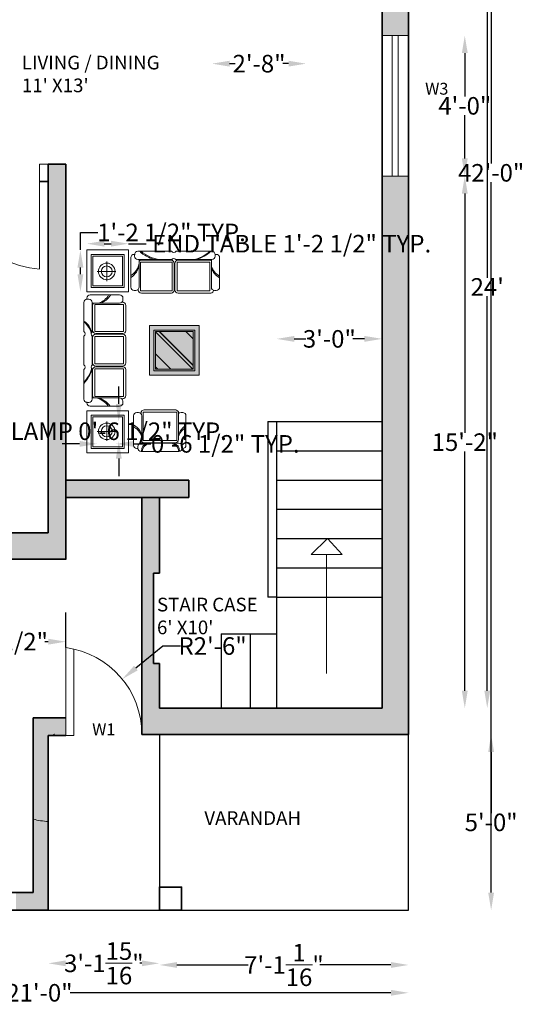
# Model space of a CAD drawing. Units: inches. Extents: x 2178 to 3409, y 1711 to 2279.
# Tile 2 of 8: x 2343 to 2516, y 1711 to 2047. Entities that reach past the tile are written whole.
import ezdxf

# ---------------------------------------------------------------- set-up
doc = ezdxf.new("R2010")
doc.units = ezdxf.units.IN
doc.linetypes.add('ACAD_ISO03W100', pattern=[30, 12, -18])
for name, color, linetype, lineweight in [('A-ANNO-DIMS', 2, 'Continuous', 18), ('A-ANNO-IDEN', 3, 'Continuous', 18), ('A-ANNO-SYMB', 7, 'Continuous', 18), ('A-AREA-IDEN', 7, 'Continuous', 18), ('A-COLS', 7, 'Continuous', 35), ('A-DOOR', 4, 'Continuous', 18), ('A-FLOR', 7, 'Continuous', 25), ('A-FLOR-STRS', 7, 'Continuous', 25), ('A-FURN', 8, 'Continuous', 18), ('A-FURN-PATT', 9, 'Continuous', 13), ('A-GLAZ', 4, 'Continuous', 18), ('A-WALL', 7, 'Continuous', 35), ('A-WALL-HIDN', 7, 'ACAD_ISO03W100', 25), ('A-WALL-PATT', 252, 'Continuous', 13)]:
    doc.layers.add(name, color=color, linetype=linetype, lineweight=lineweight)
doc.styles.get("Standard").update_dxf_attribs({"font": 'arial.ttf'})
doc.dimstyles.get("Standard").update_dxf_attribs({"dimtxt": 6, "dimasz": 6, "dimexe": 0.18, "dimexo": 0.0625, "dimgap": 0.09, "dimtad": 0, "dimtih": 1, "dimtoh": 1, "dimdec": 4, "dimzin": 0, "dimdsep": 46, "dimlunit": 4, "dimtxsty": 'Standard', "dimcen": 0.09, "dimse1": 1, "dimse2": 1, "dimadec": 0, "dimazin": 0, "dimtfac": 1, "dimtdec": 4, "dimtofl": 0, "dimtmove": 0, "dimatfit": 3, "dimfxl": 1, "dimtolj": 1, "dimtzin": 0, "dimarcsym": 0})

# ---------------------------------------------------------------- blocks, each defined once
blk = doc.blocks.new('*D17')
at = {"layer": 'A-ANNO-DIMS', "color": 0, "lineweight": -2, "transparency": 16777216}
for p, q in [((2359.06, 1724.86), (2359.75, 1724.86)), ((2385.03, 1724.86), (2384.35, 1724.86))]:
    blk.add_line(p, q, dxfattribs=at)
at = {"layer": 'A-ANNO-DIMS', "color": 0, "transparency": 16777216}
for points in [[(2359.06, 1725.86), (2359.06, 1723.86), (2353.06, 1724.86)], [(2385.03, 1725.86), (2385.03, 1723.86), (2391.03, 1724.86)]]:
    blk.add_solid(points, dxfattribs=at)
at = {"layer": 'Defpoints', "color": 0, "transparency": 16777216}
for p in [(2353.06, 1743.04), (2391.03, 1743.04), (2391.03, 1724.86)]:
    blk.add_point(p, dxfattribs=at)
at = {"layer": 'A-ANNO-DIMS', "color": 0, "transparency": 16777216, "insert": (2372.05, 1724.86), "char_height": 6, "attachment_point": 5}
blk.add_mtext('\\A1;3\'-1{\\H1x;\\S15/16;}"', dxfattribs=at)
blk = doc.blocks.new('*D18')
at = {"layer": 'A-ANNO-DIMS', "color": 0, "lineweight": -2, "transparency": 16777216}
for p, q in [((2397.03, 1724.3), (2421.29, 1724.3)), ((2470.06, 1724.3), (2445.8, 1724.3))]:
    blk.add_line(p, q, dxfattribs=at)
at = {"layer": 'A-ANNO-DIMS', "color": 0, "transparency": 16777216}
for points in [[(2397.03, 1725.3), (2397.03, 1723.3), (2391.03, 1724.3)], [(2470.06, 1725.3), (2470.06, 1723.3), (2476.06, 1724.3)]]:
    blk.add_solid(points, dxfattribs=at)
at = {"layer": 'Defpoints', "color": 0, "transparency": 16777216}
for p in [(2391.03, 1743.04), (2476.06, 1743.04), (2476.06, 1724.3)]:
    blk.add_point(p, dxfattribs=at)
at = {"layer": 'A-ANNO-DIMS', "color": 0, "transparency": 16777216, "insert": (2433.55, 1724.3), "char_height": 6, "attachment_point": 5}
blk.add_mtext('\\A1;7\'-1{\\H1x;\\S1/16;}"', dxfattribs=at)
blk = doc.blocks.new('*D22')
at = {"layer": 'A-ANNO-DIMS', "color": 0, "lineweight": -2, "transparency": 16777216}
for p, q in [((2502.98, 2094.04), (2502.98, 1959.14)), ((2502.98, 1818.04), (2502.98, 1952.94))]:
    blk.add_line(p, q, dxfattribs=at)
at = {"layer": 'A-ANNO-DIMS', "color": 0, "transparency": 16777216}
for points in [[(2501.98, 2094.04), (2503.98, 2094.04), (2502.98, 2100.04)], [(2501.98, 1818.04), (2503.98, 1818.04), (2502.98, 1812.04)]]:
    blk.add_solid(points, dxfattribs=at)
at = {"layer": 'Defpoints', "color": 0, "transparency": 16777216}
for p in [(2467.06, 2100.04), (2467.06, 1812.04), (2502.98, 1812.04)]:
    blk.add_point(p, dxfattribs=at)
at = {"layer": 'A-ANNO-DIMS', "color": 0, "transparency": 16777216, "insert": (2502.98, 1956.04), "char_height": 6, "attachment_point": 5}
blk.add_mtext("\\A1;24'", dxfattribs=at)
blk = doc.blocks.new('END-TABLE')
for p, q in [((14.32, 14.32), (0, 14.32)), ((0, 14.32), (0, 0)), ((14.32, 0), (14.32, 14.32)), ((12.81, 12.81), (1.51, 12.81)), ((1.51, 12.81), (1.51, 1.51)), ((12.25, 12.25), (2.07, 12.25)), ((2.07, 12.25), (2.07, 2.07)), ((12.25, 2.07), (12.25, 12.25)), ((12.81, 1.51), (12.81, 12.81)), ((0, 0), (14.32, 0)), ((1.51, 1.51), (12.81, 1.51)), ((2.07, 2.07), (12.25, 2.07))]:
    blk.add_line(p, q)
blk = doc.blocks.new('TABLE-LAMP')
for p, q in [((3.28, 0), (3.28, 6.65)), ((0, 3.28), (6.38, 3.28))]:
    blk.add_line(p, q)
for radius in [2.83, 1.88]:
    blk.add_circle((3.28, 3.28), radius)
blk = doc.blocks.new('DOOR-36')
for p, q in [((0, 0), (0, 36)), ((3, 0), (3, 35.87)), ((3, 0), (0, 0))]:
    blk.add_line(p, q)
blk.add_arc((0, 0), 36, 0, 85.2198)
blk = doc.blocks.new('*D43')
at = {"layer": 'A-ANNO-DIMS', "color": 0, "lineweight": -2, "transparency": 16777216}
for p, q in [((2372.2, 1970.82), (2374.52, 1970.82)), ((2380.52, 1970.82), (2386.52, 1970.82))]:
    blk.add_line(p, q, dxfattribs=at)
at = {"layer": 'A-ANNO-DIMS', "color": 0, "transparency": 16777216}
for points in [[(2372.2, 1971.82), (2372.2, 1969.82), (2366.2, 1970.82)], [(2374.52, 1971.82), (2374.52, 1969.82), (2380.52, 1970.82)]]:
    blk.add_solid(points, dxfattribs=at)
at = {"layer": 'Defpoints', "color": 0, "transparency": 16777216}
for p in [(2366.2, 1968.67), (2380.52, 1970.82), (2380.52, 1968.67)]:
    blk.add_point(p, dxfattribs=at)
at = {"layer": 'A-ANNO-DIMS', "color": 0, "transparency": 16777216, "insert": (2436.18, 1970.82), "char_height": 6, "attachment_point": 5}
blk.add_mtext('\\A1;END TABLE 1\'-2 1/2" TYP.', dxfattribs=at)
blk = doc.blocks.new('*D44')
at = {"layer": 'A-ANNO-DIMS', "color": 0, "lineweight": -2, "transparency": 16777216}
for p, q in [((2364.05, 1968.67), (2364.05, 1974.67)), ((2364.05, 1974.67), (2370.05, 1974.67)), ((2364.05, 1960.35), (2364.05, 1962.67))]:
    blk.add_line(p, q, dxfattribs=at)
at = {"layer": 'A-ANNO-DIMS', "color": 0, "transparency": 16777216}
for points in [[(2363.05, 1962.67), (2365.05, 1962.67), (2364.05, 1968.67)], [(2363.05, 1960.35), (2365.05, 1960.35), (2364.05, 1954.35)]]:
    blk.add_solid(points, dxfattribs=at)
at = {"layer": 'Defpoints', "color": 0, "transparency": 16777216}
for p in [(2364.05, 1968.67), (2366.2, 1968.67), (2366.2, 1954.35)]:
    blk.add_point(p, dxfattribs=at)
at = {"layer": 'A-ANNO-DIMS', "color": 0, "transparency": 16777216, "insert": (2395.14, 1974.67), "char_height": 6, "attachment_point": 5}
blk.add_mtext('\\A1;1\'-2 1/2" TYP.', dxfattribs=at)
blk = doc.blocks.new('*D45')
at = {"layer": 'A-ANNO-DIMS', "color": 0, "lineweight": -2, "transparency": 16777216}
for p, q in [((2377.15, 1916.05), (2377.15, 1922.05)), ((2377.15, 1897.4), (2377.15, 1891.4))]:
    blk.add_line(p, q, dxfattribs=at)
at = {"layer": 'A-ANNO-DIMS', "color": 0, "transparency": 16777216}
for points in [[(2376.15, 1916.05), (2378.15, 1916.05), (2377.15, 1910.05)], [(2376.15, 1897.4), (2378.15, 1897.4), (2377.15, 1903.4)]]:
    blk.add_solid(points, dxfattribs=at)
at = {"layer": 'Defpoints', "color": 0, "transparency": 16777216}
for p in [(2376.15, 1910.05), (2377.15, 1910.05), (2376.15, 1903.4)]:
    blk.add_point(p, dxfattribs=at)
at = {"layer": 'A-ANNO-DIMS', "color": 0, "transparency": 16777216, "insert": (2377.15, 1906.72), "char_height": 6, "attachment_point": 5}
blk.add_mtext('\\A1;LAMP 0\'-6 1/2" TYP.', dxfattribs=at)
blk = doc.blocks.new('*D46')
at = {"layer": 'A-ANNO-DIMS', "color": 0, "lineweight": -2, "transparency": 16777216}
for p, q in [((2363.77, 1902.4), (2357.77, 1902.4)), ((2382.15, 1902.4), (2388.15, 1902.4))]:
    blk.add_line(p, q, dxfattribs=at)
at = {"layer": 'A-ANNO-DIMS', "color": 0, "transparency": 16777216}
for points in [[(2363.77, 1903.4), (2363.77, 1901.4), (2369.77, 1902.4)], [(2382.15, 1903.4), (2382.15, 1901.4), (2376.15, 1902.4)]]:
    blk.add_solid(points, dxfattribs=at)
at = {"layer": 'Defpoints', "color": 0, "transparency": 16777216}
for p in [(2369.77, 1903.4), (2376.15, 1903.4), (2376.15, 1902.4)]:
    blk.add_point(p, dxfattribs=at)
at = {"layer": 'A-ANNO-DIMS', "color": 0, "transparency": 16777216, "insert": (2413.52, 1902.4), "char_height": 6, "attachment_point": 5}
blk.add_mtext('\\A1;0\'-6 1/2" TYP.', dxfattribs=at)
blk = doc.blocks.new('*D53')
at = {"layer": 'A-ANNO-DIMS', "color": 0, "lineweight": -2, "transparency": 16777216}
for p, q in [((2293.06, 2057.04), (2311.06, 2057.04)), ((2317.06, 2057.04), (2323.06, 2057.04))]:
    blk.add_line(p, q, dxfattribs=at)
at = {"layer": 'A-ANNO-DIMS', "color": 0, "transparency": 16777216}
for points in [[(2293.06, 2058.04), (2293.06, 2056.04), (2287.06, 2057.04)], [(2311.06, 2058.04), (2311.06, 2056.04), (2317.06, 2057.04)]]:
    blk.add_solid(points, dxfattribs=at)
at = {"layer": 'Defpoints', "color": 0, "transparency": 16777216}
for p in [(2287.06, 2061.54), (2317.06, 2061.54), (2317.06, 2057.04)]:
    blk.add_point(p, dxfattribs=at)
at = {"layer": 'A-ANNO-DIMS', "color": 0, "transparency": 16777216, "insert": (2347.81, 2057.04), "char_height": 6, "attachment_point": 5}
blk.add_mtext('\\A1;D2 2\'-6" TYP.', dxfattribs=at)
blk = doc.blocks.new('*D59')
at = {"layer": 'A-ANNO-DIMS', "color": 0, "lineweight": -2, "transparency": 16777216}
for p, q in [((2495.31, 2035.94), (2495.31, 2021.09)), ((2495.31, 1999.94), (2495.31, 2014.78))]:
    blk.add_line(p, q, dxfattribs=at)
at = {"layer": 'A-ANNO-DIMS', "color": 0, "transparency": 16777216}
for points in [[(2494.31, 2035.94), (2496.31, 2035.94), (2495.31, 2041.94)], [(2494.31, 1999.94), (2496.31, 1999.94), (2495.31, 1993.94)]]:
    blk.add_solid(points, dxfattribs=at)
at = {"layer": 'Defpoints', "color": 0, "transparency": 16777216}
for p in [(2467.06, 2041.94), (2467.06, 1993.94), (2495.31, 1993.94)]:
    blk.add_point(p, dxfattribs=at)
at = {"layer": 'A-ANNO-DIMS', "color": 0, "transparency": 16777216, "insert": (2495.31, 2017.94), "char_height": 6, "attachment_point": 5}
blk.add_mtext('\\A1;4\'-0"', dxfattribs=at)
blk = doc.blocks.new('*D60')
at = {"layer": 'A-ANNO-DIMS', "color": 0, "lineweight": -2, "transparency": 16777216}
for p, q in [((2495.31, 1987.94), (2495.31, 1906.14)), ((2495.31, 1818.04), (2495.31, 1899.84))]:
    blk.add_line(p, q, dxfattribs=at)
at = {"layer": 'A-ANNO-DIMS', "color": 0, "transparency": 16777216}
for points in [[(2494.31, 1987.94), (2496.31, 1987.94), (2495.31, 1993.94)], [(2494.31, 1818.04), (2496.31, 1818.04), (2495.31, 1812.04)]]:
    blk.add_solid(points, dxfattribs=at)
at = {"layer": 'Defpoints', "color": 0, "transparency": 16777216}
for p in [(2467.06, 1993.94), (2467.06, 1812.04), (2495.31, 1812.04)]:
    blk.add_point(p, dxfattribs=at)
at = {"layer": 'A-ANNO-DIMS', "color": 0, "transparency": 16777216, "insert": (2495.31, 1902.99), "char_height": 6, "attachment_point": 5}
blk.add_mtext('\\A1;15\'-2"', dxfattribs=at)
blk = doc.blocks.new('*D66')
at = {"layer": 'A-ANNO-DIMS', "color": 0, "lineweight": -2, "transparency": 16777216}
for p, q in [((2414.97, 2032.35), (2416.94, 2032.35)), ((2435.13, 2032.35), (2433.17, 2032.35))]:
    blk.add_line(p, q, dxfattribs=at)
at = {"layer": 'A-ANNO-DIMS', "color": 0, "transparency": 16777216}
for points in [[(2414.97, 2033.35), (2414.97, 2031.35), (2408.97, 2032.35)], [(2435.13, 2033.35), (2435.13, 2031.35), (2441.13, 2032.35)]]:
    blk.add_solid(points, dxfattribs=at)
at = {"layer": 'Defpoints', "color": 0, "transparency": 16777216}
for p in [(2408.97, 2060.6), (2441.13, 2060.6), (2408.97, 2032.35)]:
    blk.add_point(p, dxfattribs=at)
at = {"layer": 'A-ANNO-DIMS', "color": 0, "transparency": 16777216, "insert": (2425.05, 2032.35), "char_height": 6, "attachment_point": 5}
blk.add_mtext('\\A1;2\'-8"', dxfattribs=at)
blk = doc.blocks.new('*D68')
at = {"layer": 'A-ANNO-DIMS', "color": 0, "lineweight": -2, "transparency": 16777216}
for p, q in [((2320.65, 1834.79), (2321.8, 1834.79)), ((2353.06, 1834.79), (2351.91, 1834.79))]:
    blk.add_line(p, q, dxfattribs=at)
at = {"layer": 'A-ANNO-DIMS', "color": 0, "transparency": 16777216}
for points in [[(2320.65, 1835.79), (2320.65, 1833.79), (2314.65, 1834.79)], [(2353.06, 1835.79), (2353.06, 1833.79), (2359.06, 1834.79)]]:
    blk.add_solid(points, dxfattribs=at)
at = {"layer": 'Defpoints', "color": 0, "transparency": 16777216}
for p in [(2314.65, 1863.04), (2359.06, 1863.04), (2314.65, 1834.79)]:
    blk.add_point(p, dxfattribs=at)
at = {"layer": 'A-ANNO-DIMS', "color": 0, "transparency": 16777216, "insert": (2336.86, 1834.79), "char_height": 6, "attachment_point": 5}
blk.add_mtext('\\A1;3\'-8 1/2"', dxfattribs=at)
blk = doc.blocks.new('*D69')
at = {"layer": 'A-ANNO-DIMS', "color": 0, "lineweight": -2, "transparency": 16777216}
for p, q in [((2437.06, 1938.29), (2441, 1938.29)), ((2461.06, 1938.29), (2457.13, 1938.29))]:
    blk.add_line(p, q, dxfattribs=at)
at = {"layer": 'A-ANNO-DIMS', "color": 0, "transparency": 16777216}
for points in [[(2437.06, 1939.29), (2437.06, 1937.29), (2431.06, 1938.29)], [(2461.06, 1939.29), (2461.06, 1937.29), (2467.06, 1938.29)]]:
    blk.add_solid(points, dxfattribs=at)
at = {"layer": 'Defpoints', "color": 0, "transparency": 16777216}
for p in [(2467.06, 1938.29), (2431.06, 1910.04), (2467.06, 1910.04)]:
    blk.add_point(p, dxfattribs=at)
at = {"layer": 'A-ANNO-DIMS', "color": 0, "transparency": 16777216, "insert": (2449.06, 1938.29), "char_height": 6, "attachment_point": 5}
blk.add_mtext('\\A1;3\'-0"', dxfattribs=at)
blk = doc.blocks.new('*D70')
at = {"layer": 'A-ANNO-DIMS', "color": 0, "lineweight": -2, "transparency": 16777216}
for p, q in [((2504.31, 1797.04), (2504.31, 1776.2)), ((2504.31, 1749.04), (2504.31, 1769.89))]:
    blk.add_line(p, q, dxfattribs=at)
at = {"layer": 'A-ANNO-DIMS', "color": 0, "transparency": 16777216}
for points in [[(2503.31, 1797.04), (2505.31, 1797.04), (2504.31, 1803.04)], [(2503.31, 1749.04), (2505.31, 1749.04), (2504.31, 1743.04)]]:
    blk.add_solid(points, dxfattribs=at)
at = {"layer": 'Defpoints', "color": 0, "transparency": 16777216}
for p in [(2476.06, 1803.04), (2504.31, 1803.04), (2476.06, 1743.04)]:
    blk.add_point(p, dxfattribs=at)
at = {"layer": 'A-ANNO-DIMS', "color": 0, "transparency": 16777216, "insert": (2504.31, 1773.04), "char_height": 6, "attachment_point": 5}
blk.add_mtext('\\A1;5\'-0"', dxfattribs=at)
blk = doc.blocks.new('*D71')
at = {"layer": 'A-ANNO-DIMS', "color": 0, "lineweight": -2, "transparency": 16777216}
for p, q in [((2381.625685, 2275.292563), (2375.625685, 2275.292563)), ((2410.582731, 2275.292563), (2416.582731, 2275.292563))]:
    blk.add_line(p, q, dxfattribs=at)
at = {"layer": 'A-ANNO-DIMS', "color": 0, "transparency": 16777216}
for points in [[(2381.625685, 2276.292563), (2381.625685, 2274.292563), (2387.625685, 2275.292563)], [(2410.582731, 2276.292563), (2410.582731, 2274.292563), (2404.582731, 2275.292563)]]:
    blk.add_solid(points, dxfattribs=at)
at = {"layer": 'Defpoints', "color": 0, "transparency": 16777216}
for p in [(2404.582731, 2275.292563), (2387.625685, 1942.827852), (2404.582731, 1942.827852)]:
    blk.add_point(p, dxfattribs=at)
at = {"layer": 'A-ANNO-DIMS', "color": 0, "transparency": 16777216, "insert": (2396.104208, 2275.292563), "char_height": 6, "attachment_point": 5}
blk.add_mtext('\\A1;1\'-5"', dxfattribs=at)
blk = doc.blocks.new('*D72')
at = {"layer": 'A-ANNO-DIMS', "color": 0, "lineweight": -2, "transparency": 16777216}
for p, q in [((2195.81, 1946.99), (2195.81, 1937.48)), ((2195.81, 1921.59), (2195.81, 1931.1))]:
    blk.add_line(p, q, dxfattribs=at)
at = {"layer": 'A-ANNO-DIMS', "color": 0, "transparency": 16777216}
for points in [[(2194.81, 1946.99), (2196.81, 1946.99), (2195.81, 1952.99)], [(2194.81, 1921.59), (2196.81, 1921.59), (2195.81, 1915.59)]]:
    blk.add_solid(points, dxfattribs=at)
at = {"layer": 'Defpoints', "color": 0, "transparency": 16777216}
for p in [(2195.81, 1952.99), (2366.59, 1952.99), (2366.59, 1915.59)]:
    blk.add_point(p, dxfattribs=at)
at = {"layer": 'A-ANNO-DIMS', "color": 0, "transparency": 16777216, "insert": (2195.81, 1934.29), "char_height": 6, "attachment_point": 5}
blk.add_mtext('\\A1;3\'-1 1/2"', dxfattribs=at)
blk = doc.blocks.new('*D73')
at = {"layer": 'A-ANNO-DIMS', "color": 0, "lineweight": -2, "transparency": 16777216}
for p, q in [((2387.37, 2275.29), (2388.32, 2275.29)), ((2405.5, 2275.29), (2404.55, 2275.29))]:
    blk.add_line(p, q, dxfattribs=at)
at = {"layer": 'A-ANNO-DIMS', "color": 0, "transparency": 16777216}
for points in [[(2387.37, 2276.29), (2387.37, 2274.29), (2381.37, 2275.29)], [(2405.5, 2276.29), (2405.5, 2274.29), (2411.5, 2275.29)]]:
    blk.add_solid(points, dxfattribs=at)
at = {"layer": 'Defpoints', "color": 0, "transparency": 16777216}
for p in [(2411.5, 2275.29), (2381.37, 1966.49), (2411.5, 1966.49)]:
    blk.add_point(p, dxfattribs=at)
at = {"layer": 'A-ANNO-DIMS', "color": 0, "transparency": 16777216, "insert": (2396.44, 2275.29), "char_height": 6, "attachment_point": 5}
blk.add_mtext('\\A1;2\'-6"', dxfattribs=at)
blk = doc.blocks.new('*D74')
at = {"layer": 'A-ANNO-DIMS', "color": 0, "lineweight": -2, "transparency": 16777216}
for p, q in [((2230.06, 1714.79), (2339.62, 1714.79)), ((2470.06, 1714.79), (2360.51, 1714.79))]:
    blk.add_line(p, q, dxfattribs=at)
at = {"layer": 'A-ANNO-DIMS', "color": 0, "transparency": 16777216}
for points in [[(2230.06, 1715.79), (2230.06, 1713.79), (2224.06, 1714.79)], [(2470.06, 1715.79), (2470.06, 1713.79), (2476.06, 1714.79)]]:
    blk.add_solid(points, dxfattribs=at)
at = {"layer": 'Defpoints', "color": 0, "transparency": 16777216}
for p in [(2224.06, 1743.04), (2476.06, 1743.04), (2476.06, 1714.79)]:
    blk.add_point(p, dxfattribs=at)
at = {"layer": 'A-ANNO-DIMS', "color": 0, "transparency": 16777216, "insert": (2350.06, 1714.79), "char_height": 6, "attachment_point": 5}
blk.add_mtext('\\A1;21\'-0"', dxfattribs=at)
blk = doc.blocks.new('*D75')
at = {"layer": 'A-ANNO-DIMS', "color": 0, "lineweight": -2, "transparency": 16777216}
for p, q in [((2504.31, 2241.04), (2504.31, 1998.2)), ((2504.31, 1749.04), (2504.31, 1991.89))]:
    blk.add_line(p, q, dxfattribs=at)
at = {"layer": 'A-ANNO-DIMS', "color": 0, "transparency": 16777216}
for points in [[(2503.31, 2241.04), (2505.31, 2241.04), (2504.31, 2247.04)], [(2503.31, 1749.04), (2505.31, 1749.04), (2504.31, 1743.04)]]:
    blk.add_solid(points, dxfattribs=at)
at = {"layer": 'Defpoints', "color": 0, "transparency": 16777216}
for p in [(2476.06, 2247.04), (2504.31, 2247.04), (2476.06, 1743.04)]:
    blk.add_point(p, dxfattribs=at)
at = {"layer": 'A-ANNO-DIMS', "color": 0, "transparency": 16777216, "insert": (2504.31, 1995.04), "char_height": 6, "attachment_point": 5}
blk.add_mtext('\\A1;42\'-0"', dxfattribs=at)
blk = doc.blocks.new('*D76')
at = {"layer": 'A-ANNO-DIMS', "color": 0, "lineweight": -2, "transparency": 16777216}
for p, q in [((2392.25, 1833.31), (2382.99, 1825.78)), ((2398.25, 1833.31), (2392.25, 1833.31)), ((2355.04, 1803.14), (2355.22, 1803.14)), ((2355.13, 1803.05), (2355.13, 1803.23))]:
    blk.add_line(p, q, dxfattribs=at)
at = {"layer": 'A-ANNO-DIMS', "color": 0, "transparency": 16777216}
blk.add_solid([(2382.36, 1826.55), (2383.62, 1825), (2378.33, 1821.99)], dxfattribs=at)
at = {"layer": 'Defpoints', "color": 0, "transparency": 16777216}
for p in [(2378.33, 1821.99), (2355.13, 1803.14)]:
    blk.add_point(p, dxfattribs=at)
at = {"layer": 'A-ANNO-DIMS', "color": 0, "transparency": 16777216, "insert": (2409.19, 1833.31), "char_height": 6, "attachment_point": 5}
blk.add_mtext('\\A1;R2\'-6"', dxfattribs=at)

msp = doc.modelspace()

# ---------------------------------------------------------------- hatches: boundary and pattern name
at = {"layer": 'A-FURN-PATT'}
h = msp.add_hatch(dxfattribs=at)
h.set_pattern_fill('CROSS', color=256, scale=0.659441, angle=135, style=0)
h.set_pattern_definition([(135, (445.20567, 702.34283), (-0.233147488, 0), [0.082430085, -0.247290254]), (225, (445.20567, 702.40111), (0, -0.233147488), [0.082430085, -0.247290254])])
h.paths.add_polyline_path([(2404.58273, 1942.82785), (2387.62569, 1942.82785), (2387.62569, 1925.87081), (2404.58273, 1925.87081)])
h = msp.add_hatch(dxfattribs=at)
h.set_pattern_fill('AR-RROOF', color=256, scale=9.420581, angle=135, style=0)
h.set_pattern_definition([(135, (445.206, 702.343), (-21.31634, 7.99363), [141.3087, -18.84116, 47.1029, -9.4206]), (135, (433.015, 707.872), (-2.19825, -15.52096), [28.26174, -3.1088, 56.52349, -7.06544]), (135, (436.213, 700.0114), (-39.102164, 30.175946), [75.36465, -13.18881, 37.68232, -9.42058])])
h.paths.add_polyline_path([(2402.5102, 1940.75532), (2389.69821, 1940.75532), (2389.69821, 1927.94333), (2402.5102, 1927.94333)])
at = {"layer": 'A-WALL-PATT'}
h = msp.add_hatch(color=256, dxfattribs=at)
h.dxf.hatch_style = 1
h.paths.add_polyline_path([(2233.06485, 1992.04256), (2317.06485, 1992.04256), (2317.06485, 1998.04256), (2317.06485, 2006.75072), (2311.06485, 2006.75072), (2311.06485, 1998.04256), (2233.06485, 1998.04256), (2233.06485, 2009.64251), (2224.06485, 2009.64251), (2224.06485, 1863.04256), (2233.06485, 1863.04256), (2278.65041, 1863.04256), (2278.65041, 1872.04256), (2233.06485, 1872.04256)])
h.paths.add_polyline_path([(2359.06485, 1992.04256), (2359.06485, 1998.04256), (2353.06485, 1998.04256), (2353.06485, 1962.04256), (2353.06485, 1872.04256), (2314.65041, 1872.04256), (2314.65041, 1863.04256), (2359.06485, 1863.04256), (2359.06485, 1872.04256)])
h.paths.add_polyline_path([(2401.06485, 1890.04256), (2371.06485, 1890.04256), (2359.06485, 1890.04256), (2359.06485, 1884.04256), (2371.06485, 1884.04256), (2377.06485, 1884.04256), (2401.06485, 1884.04256)])
h.paths.add_polyline_path([(2353.06485, 1802.77269), (2359.06485, 1802.77269), (2359.06485, 1808.77269), (2356.83755, 1808.77269), (2353.06485, 1808.77269), (2347.91295, 1808.77269), (2347.91295, 1802.77269), (2347.91295, 1749.04256), (2342.02347, 1749.04256), (2342.02347, 1743.04256), (2353.06485, 1743.04256)])
h.paths.add_polyline_path([(2476.06485, 2247.04256), (2442.91353, 2247.04256), (2442.91353, 2238.04256), (2467.06485, 2238.04256), (2467.06485, 2041.93675), (2476.06485, 2041.93675)])
h.paths.add_polyline_path([(2467.06485, 2106.04256), (2406.56133, 2106.04256, -0.04188649), (2407.06485, 2100.04256), (2467.06485, 2100.04256)])
h.paths.add_polyline_path([(2406.91353, 2247.04256), (2321.22384, 2247.04256), (2321.22384, 2238.04256), (2365.06485, 2238.04256), (2365.06485, 2106.04256), (2365.06485, 2100.04256), (2371.06485, 2100.04256), (2371.06485, 2136.04256), (2371.06485, 2238.04256), (2406.91353, 2238.04256)])
h.paths.add_polyline_path([(2285.22384, 2247.04256), (2224.06485, 2247.04256), (2224.06485, 2087.1459), (2233.06485, 2087.1459), (2233.06485, 2100.04256), (2329.06485, 2100.04256, -0.04188649), (2329.56837, 2106.04256), (2233.06485, 2106.04256), (2233.06485, 2238.04256), (2285.22384, 2238.04256)])
h.paths.add_polyline_path([(2317.06485, 2052.04256), (2317.06485, 2061.5418), (2311.06485, 2061.5418), (2311.06485, 2052.04256), (2233.06485, 2052.04256), (2233.06485, 2063.1459), (2224.06485, 2063.1459), (2224.06485, 2033.64251), (2233.06485, 2033.64251), (2233.06485, 2046.04256), (2311.06485, 2046.04256), (2311.06485, 2036.1446, -0.050382044), (2317.06485, 2036.75072), (2317.06485, 2046.04256)])
h = msp.add_hatch(color=256, dxfattribs=at)
h.dxf.hatch_style = 1
h.paths.add_polyline_path([(2391.0279, 1884.04256), (2385.0279, 1884.04256), (2385.0279, 1803.04256), (2391.0279, 1803.04256), (2476.06485, 1803.04256), (2476.06485, 1993.93675), (2467.06485, 1993.93675), (2467.06485, 1812.04256), (2391.0279, 1812.04256), (2391.0279, 1827.33952), (2389.0279, 1827.33952), (2389.0279, 1858.18852), (2391.0279, 1858.18852)])

# ---------------------------------------------------------------- linework, layer by layer
at = {"layer": 'A-ANNO-SYMB'}
for p, q in [((2442.82902, 1864.61845), (2448.4039, 1870.04256)), ((2448.4039, 1870.04256), (2453.48941, 1864.61845)), ((2447.47373, 1864.61845), (2442.82902, 1864.61845)), ((2453.48941, 1864.61845), (2447.47373, 1864.61845)), ((2448.13468, 1823.94823), (2448.13468, 1864.61845)), ((2448.13468, 1864.61845), (2453.48941, 1864.61845))]:
    msp.add_line(p, q, dxfattribs=at)
at = {"layer": 'A-COLS'}
msp.add_lwpolyline([(2391.0279, 1743.04256), (2398.58202, 1743.04256), (2398.58202, 1750.89347), (2391.0279, 1750.89347)], close=True, dxfattribs=at)
at = {"layer": 'A-DOOR'}
for p, q in [((2359.06485, 1802.77269), (2359.06485, 1832.77269)), ((2359.06485, 1832.77269), (2359.06485, 1802.77269)), ((2359.06485, 1832.77269), (2359.06485, 1802.77269)), ((2361.81485, 1832.26422), (2361.81485, 1802.77269)), ((2361.81485, 1802.77269), (2359.06485, 1802.77269))]:
    msp.add_line(p, q, dxfattribs=at)
for start, end in [(359.8175446, 82.4432998), (256.0229114, 266.0320676)]:
    msp.add_arc((2355.13349, 1803.13776), 29.89456, start, end, dxfattribs=at)
at = {"layer": 'A-FLOR'}
for p, q in [((2391.0279, 1803.04256), (2391.0279, 1743.04256)), ((2476.06485, 1743.04256), (2476.06485, 1803.04256)), ((2353.06485, 1743.04256), (2476.06485, 1743.04256))]:
    msp.add_line(p, q, dxfattribs=at)
at = {"layer": 'A-FLOR-STRS'}
for p, q in [((2428.06485, 1910.04256), (2428.06485, 1850.04256)), ((2428.06485, 1910.04256), (2431.06485, 1910.04256)), ((2431.06485, 1910.04256), (2431.06485, 1812.04256)), ((2431.06485, 1910.04256), (2467.06485, 1910.04256)), ((2431.06485, 1900.04256), (2467.06485, 1900.04256)), ((2431.06485, 1890.04256), (2467.06485, 1890.04256)), ((2431.06485, 1880.04256), (2467.06485, 1880.04256)), ((2431.06485, 1870.04256), (2467.06485, 1870.04256)), ((2431.06485, 1860.04256), (2467.06485, 1860.04256)), ((2431.06485, 1850.04256), (2428.06485, 1850.04256)), ((2431.06485, 1850.04256), (2467.06485, 1850.04256)), ((2412.06485, 1837.42743), (2431.06485, 1837.42743)), ((2412.06485, 1837.42743), (2412.06485, 1812.04256)), ((2422.06485, 1837.42743), (2422.06485, 1812.04256))]:
    msp.add_line(p, q, dxfattribs=at)
at = {"layer": 'A-FURN'}
for p, q in [((2381.2851, 1955.99232), (2381.2851, 1966.04786)), ((2382.77639, 1967.17833), (2382.41557, 1967.17833)), ((2382.56274, 1967.08219), (2382.56274, 1966.51696)), ((2395.15439, 1968.21266), (2383.6932, 1968.21266)), ((2395.22257, 1965.38649), (2383.6932, 1965.38649)), ((2384.11127, 1955.99232), (2384.11127, 1965.46664)), ((2408.92496, 1965.38649), (2396.67292, 1965.38649)), ((2408.85678, 1968.21266), (2396.74111, 1968.21266)), ((2408.76423, 1955.99232), (2408.76423, 1965.40045)), ((2410.07181, 1967.08219), (2410.07181, 1966.51696)), ((2410.09911, 1967.17833), (2410.45994, 1967.17833)), ((2411.59041, 1955.99232), (2411.59041, 1966.04786)), ((2384.58307, 1954.73222), (2384.58307, 1964.46734)), ((2384.58307, 1964.46734), (2395.34995, 1964.46734)), ((2394.92504, 1965.23171), (2384.93783, 1965.23171)), ((2395.34995, 1964.46734), (2395.34995, 1954.73222)), ((2396.05551, 1964.10124), (2396.05551, 1954.86907)), ((2396.3133, 1964.10124), (2396.3133, 1955.05748)), ((2397.08901, 1954.73222), (2397.08901, 1964.46734)), ((2397.08901, 1964.46734), (2408.21179, 1964.46734)), ((2408.19298, 1965.23171), (2397.44377, 1965.23171)), ((2408.21179, 1964.46734), (2408.21179, 1954.73222)), ((2383.80736, 1955.23439), (2383.80736, 1955.05748)), ((2366.26217, 1951.82581), (2366.26217, 1952.18663)), ((2377.44818, 1953.3171), (2367.39264, 1953.3171)), ((2378.57865, 1951.6214), (2378.57865, 1952.18663)), ((2382.9808, 1954.86185), (2382.41557, 1954.86185)), ((2395.34995, 1954.73222), (2384.58307, 1954.73222)), ((2395.11345, 1953.92701), (2384.93783, 1953.92701)), ((2408.21179, 1954.73222), (2397.08901, 1954.73222)), ((2408.57147, 1953.92701), (2397.44377, 1953.92701)), ((2409.51352, 1954.92806), (2409.51352, 1954.86907)), ((2409.8947, 1954.86185), (2410.45994, 1954.86185)), ((2365.22784, 1950.70618), (2365.22784, 1940.78192)), ((2366.35831, 1951.83665), (2366.92354, 1951.83665)), ((2377.44818, 1950.49093), (2367.97387, 1950.49093)), ((2368.05401, 1950.70618), (2368.05401, 1940.71374)), ((2368.20879, 1941.23951), (2368.20879, 1949.66437)), ((2378.70829, 1950.01914), (2368.97316, 1950.01914)), ((2368.97316, 1950.01914), (2368.97316, 1940.8146)), ((2378.21939, 1950.79484), (2378.38302, 1950.79484)), ((2378.70829, 1940.8146), (2378.70829, 1950.01914)), ((2379.51349, 1941.0511), (2379.51349, 1949.66437)), ((2404.58273, 1942.82785), (2387.62569, 1942.82785)), ((2387.62569, 1942.82785), (2387.62569, 1925.87081)), ((2404.58273, 1925.87081), (2404.58273, 1942.82785)), ((2365.22784, 1939.19521), (2365.22784, 1929.41403)), ((2368.05401, 1939.26339), (2368.05401, 1929.34585)), ((2368.20879, 1938.72149), (2368.20879, 1930.1167)), ((2368.97316, 1940.8146), (2378.70829, 1940.8146)), ((2368.97316, 1939.1464), (2378.70829, 1939.1464)), ((2368.97316, 1929.76193), (2368.97316, 1939.1464)), ((2369.33926, 1940.10904), (2378.57143, 1940.10904)), ((2369.33926, 1939.85196), (2378.57143, 1939.85196)), ((2378.70829, 1939.1464), (2378.70829, 1929.76193)), ((2379.51349, 1938.9099), (2379.51349, 1930.1167)), ((2403.07544, 1941.32056), (2389.13298, 1941.32056)), ((2389.13298, 1941.32056), (2389.13298, 1927.3781)), ((2402.5102, 1940.75532), (2389.69821, 1940.75532)), ((2389.69821, 1940.75532), (2389.69821, 1927.94333)), ((2402.5102, 1927.94333), (2402.5102, 1940.75532)), ((2403.07544, 1927.3781), (2403.07544, 1941.32056)), ((2378.70829, 1929.76193), (2368.97316, 1929.76193)), ((2369.33926, 1928.98623), (2378.38302, 1928.98623)), ((2369.33926, 1928.72844), (2378.57143, 1928.72844)), ((2365.22784, 1927.82731), (2365.22784, 1917.66989)), ((2368.05401, 1927.8955), (2368.05401, 1917.66989)), ((2368.20879, 1927.59797), (2368.20879, 1918.91451)), ((2368.97316, 1928.02288), (2378.70829, 1928.02288)), ((2368.97316, 1918.55975), (2368.97316, 1928.02288)), ((2378.70829, 1928.02288), (2378.70829, 1918.55975)), ((2379.51349, 1927.78638), (2379.51349, 1918.91451)), ((2387.62569, 1925.87081), (2404.58273, 1925.87081)), ((2389.13298, 1927.3781), (2403.07544, 1927.3781)), ((2389.69821, 1927.94333), (2402.5102, 1927.94333)), ((2378.70829, 1918.55975), (2368.97316, 1918.55975)), ((2366.26217, 1916.75307), (2366.26217, 1916.39225)), ((2366.35831, 1916.53942), (2366.92354, 1916.53942)), ((2377.44818, 1915.26178), (2367.39264, 1915.26178)), ((2377.44818, 1918.08795), (2367.97387, 1918.08795)), ((2378.20612, 1917.78404), (2378.38302, 1917.78404)), ((2378.57865, 1916.95748), (2378.57865, 1916.39225)), ((2382.22452, 1911.9948), (2382.22452, 1901.93926)), ((2383.92022, 1913.12527), (2383.35499, 1913.12527)), ((2384.74678, 1912.76601), (2384.74678, 1912.92964)), ((2385.05069, 1911.9948), (2385.05069, 1902.52049)), ((2397.00852, 1913.25491), (2385.52249, 1913.25491)), ((2385.52249, 1913.25491), (2385.52249, 1903.51978)), ((2396.61992, 1914.06011), (2385.87725, 1914.06011)), ((2397.00852, 1903.51978), (2397.00852, 1913.25491)), ((2397.56198, 1903.88588), (2397.56198, 1913.11805)), ((2398.4059, 1913.12527), (2398.97114, 1913.12527)), ((2400.10161, 1911.9948), (2400.10161, 1901.93926)), ((2383.70497, 1900.90493), (2383.70497, 1901.47017)), ((2384.83544, 1902.60064), (2397.6935, 1902.60064)), ((2385.52249, 1903.51978), (2397.00852, 1903.51978)), ((2396.43151, 1902.75541), (2385.87725, 1902.75541)), ((2398.82397, 1900.90493), (2398.82397, 1901.47017)), ((2383.71581, 1900.80879), (2383.35499, 1900.80879)), ((2384.83544, 1899.77446), (2397.6935, 1899.77446)), ((2398.82397, 1900.80879), (2398.97114, 1900.80879))]:
    msp.add_line(p, q, dxfattribs=at)
for centre, radius, start, end in [((2382.41557, 1966.04786), 1.13047, 90, 180), ((2383.6932, 1967.08219), 1.13047, 90, 180), ((2383.6932, 1966.51696), 1.13047, 180, 270), ((2392.32686, 1976.73942), 11.71559, 226.7033204, 254.9108489), ((2392.98558, 1978.29933), 13.03782, 230.3907627, 262.0602504), ((2395.94775, 1968.77874), 0.97461, 215.50856, 324.49144), ((2395.94775, 1964.73535), 0.97461, 41.9206973, 138.0793027), ((2401.03069, 1975.31473), 10.06217, 279.35882, 315.4424582), ((2400.54694, 1976.73942), 11.71559, 285.0891511, 313.2966796), ((2408.94134, 1967.08219), 1.13047, 0, 90), ((2408.94134, 1966.51696), 1.13047, 270, 0), ((2410.45994, 1966.04786), 1.13047, 0, 90), ((2377.97163, 1965.14735), 6.21202, 302.2352052, 351.9364077), ((2377.97163, 1964.51911), 6.21202, 302.2352052, 351.9364077), ((2384.93783, 1964.10124), 1.13047, 90, 136.9838581), ((2394.92504, 1964.10124), 1.13047, 0, 90), ((2397.44377, 1964.10124), 1.13047, 90, 180), ((2408.21871, 1964.59092), 0.6413, 31.7185097, 92.2998875), ((2414.64403, 1965.14735), 6.21202, 198.8232285, 239.8897989), ((2414.64403, 1964.51911), 6.21202, 198.8232285, 239.8897989), ((2382.41557, 1955.99232), 1.13047, 180, 270), ((2382.9808, 1956.0056), 1.13047, 270, 0), ((2409.8947, 1955.99232), 1.13047, 180, 270), ((2410.45994, 1955.99232), 1.13047, 270, 0), ((2367.39264, 1952.18663), 1.13047, 90, 180), ((2368.29316, 1956.37072), 6.21202, 288.8232284, 329.8897989), ((2368.9214, 1956.37072), 6.21202, 288.8232284, 329.8897989), ((2377.44818, 1952.18663), 1.13047, 0, 90), ((2384.93783, 1955.05748), 1.13047, 180, 270), ((2395.11345, 1954.86907), 0.94206, 270, 0), ((2397.44377, 1955.05748), 1.13047, 180, 270), ((2408.57147, 1954.86907), 0.94206, 270, 0), ((2366.35831, 1950.70618), 1.13047, 90, 180), ((2366.92354, 1950.70618), 1.13047, 0, 90), ((2369.33926, 1949.66437), 1.13047, 133.016142, 180), ((2377.44818, 1951.6214), 1.13047, 270, 0), ((2378.38302, 1949.66437), 1.13047, 0, 90), ((2360.8182, 1938.47876), 7.1418, 13.8700854, 51.2300582), ((2362.00331, 1939.27177), 6.02901, 12.0983755, 55.7660865), ((2364.66176, 1939.98857), 0.97461, 305.50856, 54.49144), ((2368.70515, 1939.98857), 0.97461, 131.9206972, 228.0793028), ((2369.33926, 1941.23951), 1.13047, 180, 270), ((2369.33926, 1938.72149), 1.13047, 90, 180), ((2378.57143, 1941.0511), 0.94206, 270, 0), ((2378.57143, 1938.9099), 0.94206, 0, 90), ((2364.66176, 1928.62067), 0.97461, 305.50856, 54.49144), ((2368.70515, 1928.62067), 0.97461, 131.9206972, 228.0793028), ((2369.33926, 1930.1167), 1.13047, 180, 270), ((2369.33926, 1927.59797), 1.13047, 90, 180), ((2378.38302, 1930.1167), 1.13047, 270, 0), ((2378.57143, 1927.78638), 0.94206, 0, 90), ((2358.12577, 1930.60477), 10.06217, 314.5575416, 346.4540441), ((2356.70109, 1931.08852), 11.71559, 316.7033206, 344.910849), ((2369.33926, 1918.91451), 1.13047, 180, 226.983858), ((2378.38302, 1918.91451), 1.13047, 270, 0), ((2366.35831, 1917.66989), 1.13047, 180, 270), ((2367.39264, 1916.39225), 1.13047, 180, 270), ((2366.92354, 1917.66989), 1.13047, 270, 0), ((2368.29316, 1911.94831), 6.21202, 32.2352053, 81.9364077), ((2368.9214, 1911.94831), 6.21202, 32.2352053, 81.9364077), ((2377.43491, 1916.95748), 1.13047, 0, 90), ((2377.44818, 1916.39225), 1.13047, 270, 0), ((2383.35499, 1911.9948), 1.13047, 90, 180), ((2383.92022, 1911.9948), 1.13047, 0, 90), ((2385.87725, 1912.92964), 1.13047, 90, 180), ((2396.44887, 1912.92964), 1.13047, 0, 90), ((2398.4059, 1911.98153), 1.13047, 90, 138.2900186), ((2398.97114, 1911.9948), 1.13047, 0, 90), ((2379.1709, 1903.46802), 6.21202, 8.0635923, 59.8897989), ((2379.1709, 1902.83978), 6.21202, 8.0635923, 59.8897989), ((2403.41507, 1903.46802), 6.21202, 122.2352052, 160.4278708), ((2403.41507, 1902.83978), 6.21202, 122.2352052, 160.4278708), ((2383.35499, 1901.93926), 1.13047, 180, 270), ((2384.83544, 1901.47017), 1.13047, 90, 180), ((2387.46488, 1900.06218), 2.56683, 103.377287, 182.6905421), ((2385.87725, 1903.88588), 1.13047, 223.0161419, 270), ((2388.1104, 1899.55514), 3.01348, 105.8072024, 174.6335765), ((2394.67828, 1899.55514), 3.01348, 5.3664235, 74.1927976), ((2395.3238, 1900.06218), 2.56683, 357.3094579, 76.622713), ((2396.43151, 1903.88588), 1.13047, 270, 0), ((2397.6935, 1901.47017), 1.13047, 0, 90), ((2398.97114, 1901.93926), 1.13047, 270, 0), ((2384.83544, 1900.90493), 1.13047, 180, 270), ((2397.6935, 1900.90493), 1.13047, 270, 0)]:
    msp.add_arc(centre, radius, start, end, dxfattribs=at)
at = {"layer": 'A-GLAZ'}
for p, q in [((2467.06485, 2041.93675), (2467.06485, 1993.93675)), ((2476.06485, 2041.93675), (2467.06485, 2041.93675)), ((2470.56485, 2041.93675), (2470.56485, 1993.93675)), ((2472.56485, 2041.93675), (2472.56485, 1993.93675)), ((2476.06485, 1993.93675), (2476.06485, 2041.93675)), ((2467.06485, 1993.93675), (2476.06485, 1993.93675))]:
    msp.add_line(p, q, dxfattribs=at)
at = {"layer": 'A-WALL'}
for p, q in [((2476.06485, 2247.04256), (2476.06485, 1803.04256)), ((2467.06485, 2238.04256), (2467.06485, 1812.04256)), ((2353.06485, 1992.04256), (2353.06485, 1998.04256)), ((2353.06485, 1998.04256), (2359.06485, 1998.04256)), ((2359.06485, 1998.04256), (2359.06485, 1992.04256)), ((2353.06485, 1992.04256), (2350.06485, 1992.04256)), ((2353.06485, 1992.04256), (2353.06485, 1872.04256)), ((2359.06485, 1992.04256), (2359.06485, 1872.04256)), ((2371.06485, 1890.04256), (2359.06485, 1890.04256)), ((2371.06485, 1890.04256), (2401.06485, 1890.04256)), ((2401.06485, 1884.04256), (2401.06485, 1890.04256)), ((2371.06485, 1884.04256), (2359.06485, 1884.04256)), ((2371.06485, 1884.04256), (2377.06485, 1884.04256)), ((2377.06485, 1884.04256), (2401.06485, 1884.04256)), ((2377.06485, 1884.04256), (2401.06485, 1884.04256)), ((2385.0279, 1858.18852), (2385.0279, 1884.04256)), ((2385.0279, 1884.04256), (2385.0279, 1803.04256)), ((2385.0279, 1884.04256), (2391.0279, 1884.04256)), ((2391.0279, 1858.18852), (2391.0279, 1884.04256)), ((2233.06485, 1872.04256), (2353.06485, 1872.04256)), ((2359.06485, 1872.04256), (2359.06485, 1863.04256)), ((2233.06485, 1863.04256), (2359.06485, 1863.04256)), ((2389.0279, 1858.18852), (2389.0279, 1827.33952)), ((2389.0279, 1858.18852), (2391.0279, 1858.18852)), ((2389.0279, 1827.33952), (2391.0279, 1827.33952)), ((2391.0279, 1812.04256), (2391.0279, 1827.33952)), ((2391.0279, 1812.04256), (2467.06485, 1812.04256)), ((2347.91295, 1802.77269), (2347.91295, 1808.77269)), ((2347.91295, 1808.77269), (2353.06485, 1808.77269)), ((2353.06485, 1808.77269), (2356.83755, 1808.77269)), ((2356.83755, 1808.77269), (2359.06485, 1808.77269)), ((2347.91295, 1749.04256), (2347.91295, 1802.77269)), ((2353.06485, 1743.04256), (2353.06485, 1802.77269)), ((2353.06485, 1802.77269), (2359.06485, 1802.77269)), ((2385.0279, 1803.04256), (2391.0279, 1803.04256)), ((2391.0279, 1803.04256), (2476.06485, 1803.04256)), ((2467.06485, 1803.04256), (2476.06485, 1803.04256)), ((2301.6348, 1749.04256), (2347.91295, 1749.04256)), ((2301.6348, 1743.04256), (2353.06485, 1743.04256))]:
    msp.add_line(p, q, dxfattribs=at)
at = {"layer": 'A-WALL-HIDN'}
msp.add_line((2359.06485, 1832.77269), (2359.06485, 1863.04256), dxfattribs=at)

# ---------------------------------------------------------------- block references
at = {"layer": 'A-DOOR', "rotation": 180}
msp.add_blockref('DOOR-36', (2353.06485, 1998.04256), dxfattribs=at)
at = {"layer": 'A-FURN'}
for name, p in [('END-TABLE', (2366.20051, 1954.3527)), ('TABLE-LAMP', (2369.7691, 1958.06169)), ('END-TABLE', (2366.20051, 1899.35883)), ('TABLE-LAMP', (2369.7691, 1903.39516))]:
    msp.add_blockref(name, p, dxfattribs=at)

# ---------------------------------------------------------------- texts
at = {"layer": 'A-ANNO-IDEN', "char_height": 4.051205, "attachment_point": 1}
for s, insert in [('W3', (2481.78136, 2025.8057)), ('W1', (2368.0742, 1806.84048))]:
    msp.add_mtext_dynamic_manual_height_columns(s, width=167.0263497, gutter_width=20.25603, heights=[0], dxfattribs=dict(at, insert=insert))
at = {"layer": 'A-AREA-IDEN', "attachment_point": 1}
for s, insert, char_height in [("LIVING / DINING \\P11' X13'", (2344.05625, 2035.06497), 4.6796991), ("STAIR CASE\\P6' X10'", (2390.20051, 1849.81624), 4.679699), ('VARANDAH', (2406.3679, 1776.84392), 4.679699)]:
    msp.add_mtext_dynamic_manual_height_columns(s, width=123.0595467, gutter_width=23.3985, heights=[41.64659], dxfattribs=dict(at, insert=insert, char_height=char_height))

# ---------------------------------------------------------------- dimensions: what is measured, and where the dimension line sits
at = {"layer": 'A-ANNO-DIMS'}
for base, p1, p2, override, picture, middle in [((2404.58273, 2275.29256), (2387.62568, 1942.82785), (2404.58273, 1942.82785), {"dimdec": 1, "dimlfac": 1, "dimrnd": 0, "dimzin": 1, "dimdsep": 46, "dimlunit": 4, "dimfrac": 2}, '*D71', (2396.10421, 2275.29256)), ((2411.50157, 2275.29256), (2381.37394, 1966.48789), (2411.50157, 1966.48789), {"dimdec": 1, "dimlfac": 1, "dimrnd": 0, "dimzin": 1, "dimdsep": 46, "dimlunit": 4, "dimfrac": 2}, '*D73', (2396.43775, 2275.29256)), ((2467.06485, 1938.29256), (2431.06485, 1910.04256), (2467.06485, 1910.04256), {"dimdec": 1, "dimlfac": 1, "dimrnd": 0, "dimzin": 1, "dimdsep": 46, "dimlunit": 4, "dimfrac": 2}, '*D69', (2449.06485, 1938.29256)), ((2476.06485, 1714.79256), (2224.06485, 1743.04256), (2476.06485, 1743.04256), {"dimdec": 1, "dimlfac": 1, "dimrnd": 0, "dimzin": 1, "dimdsep": 46, "dimlunit": 4, "dimfrac": 2}, '*D74', (2350.06485, 1714.79256)), ((2391.027904, 1724.860777), (2353.064847, 1743.042563), (2391.027904, 1743.042563), {"dimclrd": 0, "dimclre": 0, "dimclrt": 0}, '*D17', (2372.046375, 1724.860777)), ((2476.064847, 1724.297168), (2391.027904, 1743.042563), (2476.064847, 1743.042563), {"dimclrd": 0, "dimclre": 0, "dimclrt": 0}, '*D18', (2433.546375, 1724.297168))]:
    dim = msp.add_linear_dim(base=base, p1=p1, p2=p2, dimstyle='Standard', override=override, dxfattribs=at)
    dim.commit()
    dim.dimension.update_dxf_attribs({"geometry": picture, "text_midpoint": middle})
for base, p1, p2, angle, override, picture, middle in [((2504.31485, 2247.04256), (2476.06485, 1743.04256), (2476.06485, 2247.04256), 90, {"dimdec": 1, "dimlfac": 1, "dimrnd": 0, "dimzin": 1, "dimdsep": 46, "dimlunit": 4, "dimfrac": 2}, '*D75', (2504.31485, 1995.04256)), ((2502.97839, 1812.04256), (2467.06485, 2100.04256), (2467.06485, 1812.04256), 90, {"dimclrd": 0, "dimclre": 0, "dimclrt": 0}, '*D22', (2502.97839, 1956.04256)), ((2408.97204, 2032.35384), (2441.13383, 2060.60384), (2408.97204, 2060.60384), 180, {"dimdec": 1, "dimlfac": 1, "dimrnd": 0, "dimzin": 1, "dimdsep": 46, "dimlunit": 4, "dimfrac": 2}, '*D66', (2425.05294, 2032.35384)), ((2495.31485, 1993.93675), (2467.06485, 2041.93675), (2467.06485, 1993.93675), 270, {"dimdec": 1, "dimlfac": 1, "dimrnd": 0, "dimzin": 1, "dimdsep": 46, "dimlunit": 4, "dimfrac": 2}, '*D59', (2495.31485, 2017.93675)), ((2495.31485, 1812.04256), (2467.06485, 1993.93675), (2467.06485, 1812.04256), 270, {"dimdec": 1, "dimlfac": 1, "dimrnd": 0, "dimzin": 1, "dimdsep": 46, "dimlunit": 4, "dimfrac": 2}, '*D60', (2495.31485, 1902.98966)), ((2195.81485, 1952.986), (2366.59328, 1915.59289), (2366.59328, 1952.986), 90, {"dimdec": 1, "dimlfac": 1, "dimrnd": 0, "dimzin": 1, "dimdsep": 46, "dimlunit": 4, "dimfrac": 2}, '*D72', (2195.81485, 1934.28944)), ((2314.65041, 1834.79256), (2359.06485, 1863.04256), (2314.65041, 1863.04256), 180, {"dimdec": 1, "dimlfac": 1, "dimrnd": 0, "dimzin": 1, "dimdsep": 46, "dimlunit": 4, "dimfrac": 2}, '*D68', (2336.85763, 1834.79256)), ((2504.31485, 1803.04256), (2476.06485, 1743.04256), (2476.06485, 1803.04256), 90, {"dimdec": 1, "dimlfac": 1, "dimrnd": 0, "dimzin": 1, "dimdsep": 46, "dimlunit": 4, "dimfrac": 2}, '*D70', (2504.31485, 1773.04256))]:
    dim = msp.add_linear_dim(base=base, p1=p1, p2=p2, angle=angle, dimstyle='Standard', override=override, dxfattribs=at)
    dim.commit()
    dim.dimension.update_dxf_attribs({"geometry": picture, "text_midpoint": middle})
for base, p1, p2, text, picture, middle in [((2317.06485, 2057.0418), (2287.06485, 2061.5418), (2317.06485, 2061.5418), 'D2 <> TYP.', '*D53', (2347.81378, 2057.0418)), ((2380.51979, 1970.81987), (2366.20051, 1968.67198), (2380.51979, 1968.67198), 'END TABLE <> TYP.', '*D43', (2436.18346, 1970.81987)), ((2376.14825, 1902.39728), (2369.7691, 1903.39516), (2376.14825, 1903.39516), '<> TYP.', '*D46', (2413.5152, 1902.39728))]:
    dim = msp.add_linear_dim(base=base, p1=p1, p2=p2, text=text, dimstyle='Standard', override={"dimdec": 1, "dimlfac": 1, "dimrnd": 0, "dimzin": 1, "dimdsep": 46, "dimlunit": 4, "dimfrac": 2}, dxfattribs=at)
    dim.commit()
    dim.dimension.update_dxf_attribs({"geometry": picture, "text_midpoint": middle})
for base, p1, p2, text, picture, middle in [((2364.05262, 1968.67198), (2366.20051, 1954.3527), (2366.20051, 1968.67198), '<> TYP.', '*D44', (2395.13716, 1974.67198)), ((2377.14613, 1910.04768), (2376.14825, 1903.39516), (2376.14825, 1910.04768), 'LAMP <> TYP.', '*D45', (2377.14613, 1906.72142))]:
    dim = msp.add_linear_dim(base=base, p1=p1, p2=p2, angle=90, text=text, dimstyle='Standard', override={"dimdec": 1, "dimlfac": 1, "dimrnd": 0, "dimzin": 1, "dimdsep": 46, "dimlunit": 4, "dimfrac": 2}, dxfattribs=at)
    dim.commit()
    dim.dimension.update_dxf_attribs({"geometry": picture, "text_midpoint": middle})
dim = msp.add_radius_dim(center=(2355.13349, 1803.13776), mpoint=(2378.33094, 1821.99415), dimstyle='Standard', override={"dimdec": 1, "dimlfac": 1, "dimrnd": 0, "dimzin": 1, "dimdsep": 46, "dimlunit": 4, "dimfrac": 2}, dxfattribs=at)
dim.commit()
dim.dimension.update_dxf_attribs({"geometry": '*D76', "text_midpoint": (2409.18524, 1833.30799), "dimtype": 164})

doc.saveas('drawing.dxf')
